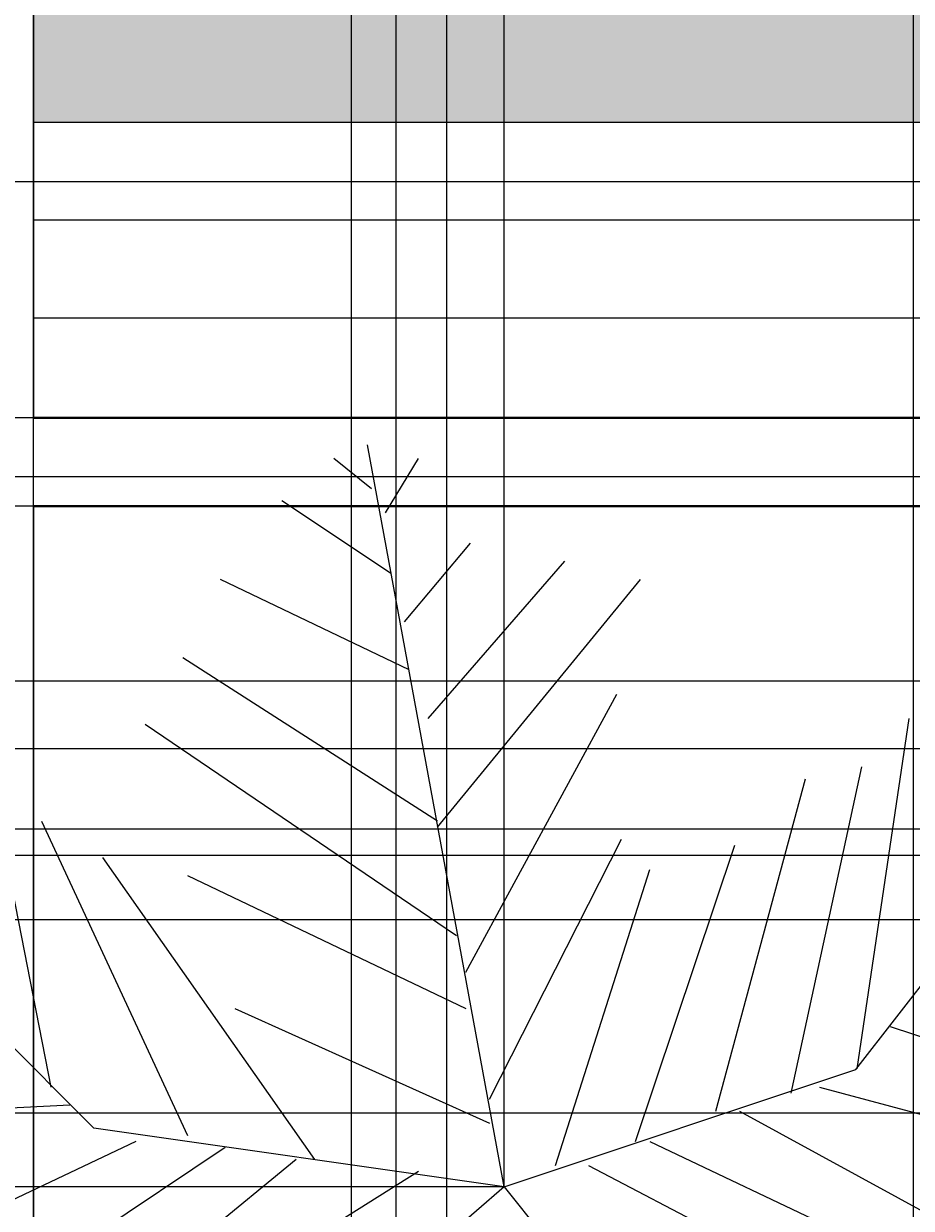
# Model space of a CAD drawing. Units: inches. Extents: x 818 to 1898, y 976 to 2364.
# Tile 64 of 96: x 1083 to 1173, y 1972 to 2093. Entities that reach past the tile are written whole.
import ezdxf

# ---------------------------------------------------------------- set-up
doc = ezdxf.new("R2010")
doc.units = ezdxf.units.IN
doc.header["$LTSCALE"] = 5
doc.header["$MEASUREMENT"] = 0
for name, color, linetype, lineweight in [('A-ANNO-DIMS', 2, 'Continuous', 18), ('A-FLOR-STRS', 7, 'Continuous', 25), ('A-WALL', 7, 'Continuous', 40), ('L-PLNT-BEDS', 94, 'Continuous', 18)]:
    doc.layers.add(name, color=color, linetype=linetype, lineweight=lineweight)
doc.layers.add('L-PLNT', color=116, linetype='Continuous', lineweight=13, true_color=0x136734)
doc.layers.add('L-PLNT-PATT', color=114, linetype='Continuous', lineweight=9, true_color=0x139b48)
doc.styles.get("Standard").update_dxf_attribs({"font": 'arial.ttf'})
doc.dimstyles.get("Standard").update_dxf_attribs({"dimtxt": 0.18, "dimasz": 0.18, "dimexe": 0.18, "dimexo": 0.0625, "dimgap": 0.09, "dimtad": 0, "dimtih": 1, "dimtoh": 1, "dimdec": 4, "dimzin": 0, "dimdsep": 46, "dimtxsty": 'Standard', "dimcen": 0.09, "dimadec": 0, "dimazin": 0, "dimtfac": 1, "dimtdec": 4, "dimtofl": 0, "dimtmove": 0, "dimatfit": 3, "dimfxl": 1, "dimtolj": 1, "dimtzin": 0, "dimarcsym": 0})

# ---------------------------------------------------------------- blocks, each defined once
blk = doc.blocks.new('PALM-DECK')
for p, q in [((74.19, 69.77), (60.24, 145.52)), ((60.66, 141.05), (56.81, 144.14)), ((62.1, 138.58), (65.47, 144.14)), ((62.58, 132.41), (51.51, 139.82)), ((64.03, 127.47), (70.77, 135.5)), ((66.43, 117.6), (80.4, 133.65)), ((64.51, 122.54), (45.25, 131.79)), ((67.4, 106.49), (88.1, 131.79)), ((67.4, 107.11), (41.4, 123.77)), ((70.29, 91.68), (85.69, 120.07)), ((110.08, 81.73), (137.98, 117.61)), ((110.24, 81.8), (115.54, 117.6)), ((69.32, 95.38), (37.55, 116.98)), ((103.5, 79.33), (110.72, 112.66)), ((95.8, 77.48), (104.95, 111.43)), ((26.96, 107.11), (41.88, 75.01)), ((72.69, 78.72), (86.17, 105.26)), ((23.11, 104.64), (27.92, 79.95)), ((87.62, 74.4), (97.73, 104.64)), ((32.33, 75.75), (4.43, 103.66)), ((54.88, 72.55), (33.22, 103.4)), ((79.43, 71.93), (89.06, 102.17)), ((41.88, 101.55), (70.29, 87.97)), ((46.7, 87.97), (72.69, 76.25)), ((113.61, 86.12), (138.16, 78.1)), ((74.19, 69.77), (110.08, 81.73)), ((106.39, 79.95), (136.24, 71.93)), ((29.85, 78.1), (4.81, 76.87)), ((98.21, 77.48), (120.83, 65.14)), ((74.19, 69.77), (32.33, 75.75)), ((36.59, 74.4), (10.59, 62.05)), ((89.06, 74.4), (115.06, 62.05)), ((45.73, 73.78), (23.59, 58.97)), ((52.96, 72.55), (34.18, 57.12)), ((82.8, 71.93), (108.8, 58.35)), ((65.47, 71.31), (45.73, 58.97)), ((74.19, 69.77), (44.29, 43.85)), ((74.19, 69.77), (98.11, 39.87))]:
    blk.add_line(p, q)
blk = doc.blocks.new('*D59')
at = {"layer": 'A-ANNO-DIMS', "color": 0, "lineweight": -2, "ltscale": 5, "transparency": 16777216}
for p, q in [((1251.64, 2300.39), (818.03, 2300.39)), ((818.21, 2300.21), (818.21, 1669.95)), ((818.21, 1039.32), (818.21, 1669.59)), ((896.05, 1039.14), (818.03, 1039.14))]:
    blk.add_line(p, q, dxfattribs=at)
at = {"layer": 'A-ANNO-DIMS', "color": 0, "ltscale": 5, "transparency": 16777216}
for points in [[(818.18, 2300.21), (818.24, 2300.21), (818.21, 2300.39)], [(818.18, 1039.32), (818.24, 1039.32), (818.21, 1039.14)]]:
    blk.add_solid(points, dxfattribs=at)
at = {"layer": 'Defpoints', "color": 0, "ltscale": 5, "transparency": 16777216}
for p in [(818.21, 2300.39), (1251.71, 2300.39), (896.11, 1039.14)]:
    blk.add_point(p, dxfattribs=at)
at = {"layer": 'A-ANNO-DIMS', "color": 0, "ltscale": 5, "transparency": 16777216, "insert": (818.21, 1669.77), "char_height": 0.18, "attachment_point": 5}
blk.add_mtext('\\A1;1261.2', dxfattribs=at)
blk = doc.blocks.new('*D61')
at = {"layer": 'A-ANNO-DIMS', "color": 0, "lineweight": -2, "ltscale": 5, "transparency": 16777216}
for p, q in [((1071.73, 1203.03), (1071.73, 2363.87)), ((1430.73, 1203.03), (1430.73, 2363.87)), ((1071.91, 2363.69), (1250.94, 2363.69)), ((1430.55, 2363.69), (1251.51, 2363.69))]:
    blk.add_line(p, q, dxfattribs=at)
at = {"layer": 'A-ANNO-DIMS', "color": 0, "ltscale": 5, "transparency": 16777216}
for points in [[(1071.91, 2363.72), (1071.91, 2363.66), (1071.73, 2363.69)], [(1430.55, 2363.72), (1430.55, 2363.66), (1430.73, 2363.69)]]:
    blk.add_solid(points, dxfattribs=at)
at = {"layer": 'Defpoints', "color": 0, "ltscale": 5, "transparency": 16777216}
for p in [(1430.73, 2363.69), (1071.73, 1202.96), (1430.73, 1202.96)]:
    blk.add_point(p, dxfattribs=at)
at = {"layer": 'A-ANNO-DIMS', "color": 0, "ltscale": 5, "transparency": 16777216, "insert": (1251.23, 2363.69), "char_height": 0.18, "attachment_point": 5}
blk.add_mtext('\\A1;359', dxfattribs=at)
blk = doc.blocks.new('*D67')
at = {"layer": 'A-ANNO-DIMS', "color": 0, "lineweight": -2, "ltscale": 5, "transparency": 16777216}
for p, q in [((1083.66, 2205.97), (818.03, 2205.97)), ((818.21, 2205.79), (818.21, 2129.71)), ((818.21, 2053.26), (818.21, 2129.34)), ((1083.66, 2053.08), (818.03, 2053.08))]:
    blk.add_line(p, q, dxfattribs=at)
at = {"layer": 'A-ANNO-DIMS', "color": 0, "ltscale": 5, "transparency": 16777216}
for points in [[(818.18, 2205.79), (818.24, 2205.79), (818.21, 2205.97)], [(818.18, 2053.26), (818.24, 2053.26), (818.21, 2053.08)]]:
    blk.add_solid(points, dxfattribs=at)
at = {"layer": 'Defpoints', "color": 0, "ltscale": 5, "transparency": 16777216}
for p in [(818.21, 2205.97), (1083.73, 2205.97), (1083.73, 2053.08)]:
    blk.add_point(p, dxfattribs=at)
at = {"layer": 'A-ANNO-DIMS', "color": 0, "ltscale": 5, "transparency": 16777216, "insert": (818.21, 2129.52), "char_height": 0.18, "attachment_point": 5}
blk.add_mtext('\\A1;152.9', dxfattribs=at)
blk = doc.blocks.new('*D73')
at = {"layer": 'A-ANNO-DIMS', "color": 0, "lineweight": -2, "ltscale": 5, "transparency": 16777216}
for p, q in [((1590.66, 2011.08), (818.03, 2011.08)), ((818.21, 2010.9), (818.21, 1996.76)), ((818.21, 1982.26), (818.21, 1996.4)), ((1590.66, 1982.08), (818.03, 1982.08))]:
    blk.add_line(p, q, dxfattribs=at)
at = {"layer": 'A-ANNO-DIMS', "color": 0, "ltscale": 5, "transparency": 16777216}
for points in [[(818.18, 2010.9), (818.24, 2010.9), (818.21, 2011.08)], [(818.18, 1982.26), (818.24, 1982.26), (818.21, 1982.08)]]:
    blk.add_solid(points, dxfattribs=at)
at = {"layer": 'Defpoints', "color": 0, "ltscale": 5, "transparency": 16777216}
for p in [(818.21, 2011.08), (1590.73, 2011.08), (1590.73, 1982.08)]:
    blk.add_point(p, dxfattribs=at)
at = {"layer": 'A-ANNO-DIMS', "color": 0, "ltscale": 5, "transparency": 16777216, "insert": (818.21, 1996.58), "char_height": 0.18, "attachment_point": 5}
blk.add_mtext('\\A1;29', dxfattribs=at)
blk = doc.blocks.new('*D82')
at = {"layer": 'A-ANNO-DIMS', "color": 0, "lineweight": -2, "ltscale": 5, "transparency": 16777216}
for p, q in [((1083.73, 1501.14), (1083.73, 2363.87)), ((1197.73, 1501.14), (1197.73, 2363.87)), ((1083.91, 2363.69), (1140.45, 2363.69)), ((1197.55, 2363.69), (1141.01, 2363.69))]:
    blk.add_line(p, q, dxfattribs=at)
at = {"layer": 'A-ANNO-DIMS', "color": 0, "ltscale": 5, "transparency": 16777216}
for points in [[(1083.91, 2363.72), (1083.91, 2363.66), (1083.73, 2363.69)], [(1197.55, 2363.72), (1197.55, 2363.66), (1197.73, 2363.69)]]:
    blk.add_solid(points, dxfattribs=at)
at = {"layer": 'Defpoints', "color": 0, "ltscale": 5, "transparency": 16777216}
for p in [(1197.73, 2363.69), (1083.73, 1501.08), (1197.73, 1501.08)]:
    blk.add_point(p, dxfattribs=at)
at = {"layer": 'A-ANNO-DIMS', "color": 0, "ltscale": 5, "transparency": 16777216, "insert": (1140.73, 2363.69), "char_height": 0.18, "attachment_point": 5}
blk.add_mtext('\\A1;114', dxfattribs=at)
blk = doc.blocks.new('*D93')
at = {"layer": 'A-ANNO-DIMS', "color": 0, "lineweight": -2, "ltscale": 5, "transparency": 16777216}
for p, q in [((1068.34, 1071.12), (1068.34, 2363.87)), ((1120.76, 1071.12), (1120.76, 2363.87)), ((1068.52, 2363.69), (1094.16, 2363.69)), ((1120.58, 2363.69), (1094.94, 2363.69))]:
    blk.add_line(p, q, dxfattribs=at)
at = {"layer": 'A-ANNO-DIMS', "color": 0, "ltscale": 5, "transparency": 16777216}
for points in [[(1068.52, 2363.72), (1068.52, 2363.66), (1068.34, 2363.69)], [(1120.58, 2363.72), (1120.58, 2363.66), (1120.76, 2363.69)]]:
    blk.add_solid(points, dxfattribs=at)
at = {"layer": 'Defpoints', "color": 0, "ltscale": 5, "transparency": 16777216}
for p in [(1120.76, 2363.69), (1068.34, 1071.06), (1120.76, 1071.06)]:
    blk.add_point(p, dxfattribs=at)
at = {"layer": 'A-ANNO-DIMS', "color": 0, "ltscale": 5, "transparency": 16777216, "insert": (1094.55, 2363.69), "char_height": 0.18, "attachment_point": 5}
blk.add_mtext('\\A1;52.42', dxfattribs=at)
blk = doc.blocks.new('*D94')
at = {"layer": 'A-ANNO-DIMS', "color": 0, "lineweight": -2, "ltscale": 5, "transparency": 16777216}
for p, q in [((1120.76, 1071.12), (1120.76, 2363.87)), ((1173.54, 1071.12), (1173.54, 2363.87)), ((1120.94, 2363.69), (1146.76, 2363.69)), ((1173.36, 2363.69), (1147.55, 2363.69))]:
    blk.add_line(p, q, dxfattribs=at)
at = {"layer": 'A-ANNO-DIMS', "color": 0, "ltscale": 5, "transparency": 16777216}
for points in [[(1120.94, 2363.72), (1120.94, 2363.66), (1120.76, 2363.69)], [(1173.36, 2363.72), (1173.36, 2363.66), (1173.54, 2363.69)]]:
    blk.add_solid(points, dxfattribs=at)
at = {"layer": 'Defpoints', "color": 0, "ltscale": 5, "transparency": 16777216}
for p in [(1173.54, 2363.69), (1120.76, 1071.06), (1173.54, 1071.06)]:
    blk.add_point(p, dxfattribs=at)
at = {"layer": 'A-ANNO-DIMS', "color": 0, "ltscale": 5, "transparency": 16777216, "insert": (1147.15, 2363.69), "char_height": 0.18, "attachment_point": 5}
blk.add_mtext('\\A1;52.78', dxfattribs=at)
blk = doc.blocks.new('*D109')
at = {"layer": 'A-ANNO-DIMS', "color": 0, "lineweight": -2, "ltscale": 5, "transparency": 16777216}
for p, q in [((1125.92, 1410.12), (1125.92, 2363.87)), ((1203.33, 1409.91), (1203.33, 2363.87)), ((1126.1, 2363.69), (1164.25, 2363.69)), ((1203.15, 2363.69), (1165, 2363.69))]:
    blk.add_line(p, q, dxfattribs=at)
at = {"layer": 'A-ANNO-DIMS', "color": 0, "ltscale": 5, "transparency": 16777216}
for points in [[(1126.1, 2363.72), (1126.1, 2363.66), (1125.92, 2363.69)], [(1203.15, 2363.72), (1203.15, 2363.66), (1203.33, 2363.69)]]:
    blk.add_solid(points, dxfattribs=at)
at = {"layer": 'Defpoints', "color": 0, "ltscale": 5, "transparency": 16777216}
for p in [(1203.33, 2363.69), (1125.92, 1410.05), (1203.33, 1409.85)]:
    blk.add_point(p, dxfattribs=at)
at = {"layer": 'A-ANNO-DIMS', "color": 0, "ltscale": 5, "transparency": 16777216, "insert": (1164.62, 2363.69), "char_height": 0.18, "attachment_point": 5}
blk.add_mtext('\\A1;77.41', dxfattribs=at)
blk = doc.blocks.new('*D123')
at = {"layer": 'A-ANNO-DIMS', "color": 0, "lineweight": -2, "ltscale": 5, "transparency": 16777216}
for p, q in [((1083.73, 2044.14), (1083.73, 2363.87)), ((1131.77, 1974.64), (1131.77, 2363.87)), ((1083.91, 2363.69), (1107.35, 2363.69)), ((1131.59, 2363.69), (1108.14, 2363.69))]:
    blk.add_line(p, q, dxfattribs=at)
at = {"layer": 'A-ANNO-DIMS', "color": 0, "ltscale": 5, "transparency": 16777216}
for points in [[(1083.91, 2363.72), (1083.91, 2363.66), (1083.73, 2363.69)], [(1131.59, 2363.72), (1131.59, 2363.66), (1131.77, 2363.69)]]:
    blk.add_solid(points, dxfattribs=at)
at = {"layer": 'Defpoints', "color": 0, "ltscale": 5, "transparency": 16777216}
for p in [(1131.77, 2363.69), (1083.73, 2044.08), (1131.77, 1974.57)]:
    blk.add_point(p, dxfattribs=at)
at = {"layer": 'A-ANNO-DIMS', "color": 0, "ltscale": 5, "transparency": 16777216, "insert": (1107.75, 2363.69), "char_height": 0.18, "attachment_point": 5}
blk.add_mtext('\\A1;48.04', dxfattribs=at)
blk = doc.blocks.new('*D124')
at = {"layer": 'A-ANNO-DIMS', "color": 0, "lineweight": -2, "ltscale": 5, "transparency": 16777216}
for p, q in [((1131.7, 1974.57), (818.03, 1974.57)), ((818.21, 1974.39), (818.21, 1884.68)), ((818.21, 1794.61), (818.21, 1884.32)), ((1138.44, 1794.43), (818.03, 1794.43))]:
    blk.add_line(p, q, dxfattribs=at)
at = {"layer": 'A-ANNO-DIMS', "color": 0, "ltscale": 5, "transparency": 16777216}
for points in [[(818.18, 1974.39), (818.24, 1974.39), (818.21, 1974.57)], [(818.18, 1794.61), (818.24, 1794.61), (818.21, 1794.43)]]:
    blk.add_solid(points, dxfattribs=at)
at = {"layer": 'Defpoints', "color": 0, "ltscale": 5, "transparency": 16777216}
for p in [(818.21, 1974.57), (1131.77, 1974.57), (1138.5, 1794.43)]:
    blk.add_point(p, dxfattribs=at)
at = {"layer": 'A-ANNO-DIMS', "color": 0, "ltscale": 5, "transparency": 16777216, "insert": (818.21, 1884.5), "char_height": 0.18, "attachment_point": 5}
blk.add_mtext('\\A1;180.14', dxfattribs=at)
blk = doc.blocks.new('*D125')
at = {"layer": 'A-ANNO-DIMS', "color": 0, "lineweight": -2, "ltscale": 5, "transparency": 16777216}
for p, q in [((1083.66, 2044.08), (818.03, 2044.08)), ((818.21, 2043.9), (818.21, 2009.51)), ((818.21, 1974.75), (818.21, 2009.14)), ((1131.7, 1974.57), (818.03, 1974.57))]:
    blk.add_line(p, q, dxfattribs=at)
at = {"layer": 'A-ANNO-DIMS', "color": 0, "ltscale": 5, "transparency": 16777216}
for points in [[(818.18, 2043.9), (818.24, 2043.9), (818.21, 2044.08)], [(818.18, 1974.75), (818.24, 1974.75), (818.21, 1974.57)]]:
    blk.add_solid(points, dxfattribs=at)
at = {"layer": 'Defpoints', "color": 0, "ltscale": 5, "transparency": 16777216}
for p in [(1083.73, 2044.08), (818.21, 1974.57), (1131.77, 1974.57)]:
    blk.add_point(p, dxfattribs=at)
at = {"layer": 'A-ANNO-DIMS', "color": 0, "ltscale": 5, "transparency": 16777216, "insert": (818.21, 2009.33), "char_height": 0.18, "attachment_point": 5}
blk.add_mtext('\\A1;69.5', dxfattribs=at)
blk = doc.blocks.new('*D126')
at = {"layer": 'A-ANNO-DIMS', "color": 0, "lineweight": -2, "ltscale": 5, "transparency": 16777216}
for p, q in [((1035.38, 1252.09), (1035.38, 2363.87)), ((1116.19, 1236.03), (1116.19, 2363.87)), ((1035.56, 2363.69), (1075.41, 2363.69)), ((1116.01, 2363.69), (1076.16, 2363.69))]:
    blk.add_line(p, q, dxfattribs=at)
at = {"layer": 'A-ANNO-DIMS', "color": 0, "ltscale": 5, "transparency": 16777216}
for points in [[(1035.56, 2363.72), (1035.56, 2363.66), (1035.38, 2363.69)], [(1116.01, 2363.72), (1116.01, 2363.66), (1116.19, 2363.69)]]:
    blk.add_solid(points, dxfattribs=at)
at = {"layer": 'Defpoints', "color": 0, "ltscale": 5, "transparency": 16777216}
for p in [(1035.38, 2363.69), (1035.38, 1252.02), (1116.19, 1235.96)]:
    blk.add_point(p, dxfattribs=at)
at = {"layer": 'A-ANNO-DIMS', "color": 0, "ltscale": 5, "transparency": 16777216, "insert": (1075.78, 2363.69), "char_height": 0.18, "attachment_point": 5}
blk.add_mtext('\\A1;80.81', dxfattribs=at)
blk = doc.blocks.new('*D140')
at = {"layer": 'A-ANNO-DIMS', "color": 0, "lineweight": -2, "ltscale": 5, "transparency": 16777216}
for p, q in [((1083.73, 2053.14), (1083.73, 2363.87)), ((1218.11, 2083.32), (1218.11, 2363.87)), ((1083.91, 2363.69), (1150.46, 2363.69)), ((1217.93, 2363.69), (1151.37, 2363.69))]:
    blk.add_line(p, q, dxfattribs=at)
at = {"layer": 'A-ANNO-DIMS', "color": 0, "ltscale": 5, "transparency": 16777216}
for points in [[(1083.91, 2363.72), (1083.91, 2363.66), (1083.73, 2363.69)], [(1217.93, 2363.72), (1217.93, 2363.66), (1218.11, 2363.69)]]:
    blk.add_solid(points, dxfattribs=at)
at = {"layer": 'Defpoints', "color": 0, "ltscale": 5, "transparency": 16777216}
for p in [(1218.11, 2363.69), (1218.11, 2083.26), (1083.73, 2053.08)]:
    blk.add_point(p, dxfattribs=at)
at = {"layer": 'A-ANNO-DIMS', "color": 0, "ltscale": 5, "transparency": 16777216, "insert": (1150.92, 2363.69), "char_height": 0.18, "attachment_point": 5}
blk.add_mtext('\\A1;134.39', dxfattribs=at)
blk = doc.blocks.new('*D146')
at = {"layer": 'A-ANNO-DIMS', "color": 0, "lineweight": -2, "ltscale": 5, "transparency": 16777216}
for p, q in [((1197.33, 2122.38), (818.03, 2122.38)), ((818.21, 2122.2), (818.21, 2087.91)), ((818.21, 2053.26), (818.21, 2087.55)), ((1083.66, 2053.08), (818.03, 2053.08))]:
    blk.add_line(p, q, dxfattribs=at)
at = {"layer": 'A-ANNO-DIMS', "color": 0, "ltscale": 5, "transparency": 16777216}
for points in [[(818.18, 2122.2), (818.24, 2122.2), (818.21, 2122.38)], [(818.18, 2053.26), (818.24, 2053.26), (818.21, 2053.08)]]:
    blk.add_solid(points, dxfattribs=at)
at = {"layer": 'Defpoints', "color": 0, "ltscale": 5, "transparency": 16777216}
for p in [(1197.39, 2122.38), (818.21, 2053.08), (1083.73, 2053.08)]:
    blk.add_point(p, dxfattribs=at)
at = {"layer": 'A-ANNO-DIMS', "color": 0, "ltscale": 5, "transparency": 16777216, "insert": (818.21, 2087.73), "char_height": 0.18, "attachment_point": 5}
blk.add_mtext('\\A1;69.3', dxfattribs=at)
blk = doc.blocks.new('*D207')
at = {"layer": 'A-ANNO-DIMS', "color": 0, "lineweight": -2, "ltscale": 5, "transparency": 16777216}
for p, q in [((1590.66, 2044.08), (818.03, 2044.08)), ((818.21, 2043.9), (818.21, 2027.76)), ((818.21, 2011.26), (818.21, 2027.4)), ((1590.66, 2011.08), (818.03, 2011.08))]:
    blk.add_line(p, q, dxfattribs=at)
at = {"layer": 'A-ANNO-DIMS', "color": 0, "ltscale": 5, "transparency": 16777216}
for points in [[(818.18, 2043.9), (818.24, 2043.9), (818.21, 2044.08)], [(818.18, 2011.26), (818.24, 2011.26), (818.21, 2011.08)]]:
    blk.add_solid(points, dxfattribs=at)
at = {"layer": 'Defpoints', "color": 0, "ltscale": 5, "transparency": 16777216}
for p in [(818.21, 2044.08), (1590.73, 2044.08), (1590.73, 2011.08)]:
    blk.add_point(p, dxfattribs=at)
at = {"layer": 'A-ANNO-DIMS', "color": 0, "ltscale": 5, "transparency": 16777216, "insert": (818.21, 2027.58), "char_height": 0.18, "attachment_point": 5}
blk.add_mtext('\\A1;33', dxfattribs=at)
blk = doc.blocks.new('*D232')
at = {"layer": 'A-ANNO-DIMS', "color": 0, "lineweight": -2, "ltscale": 5, "transparency": 16777216}
for p, q in [((1303.87, 2008.39), (818.03, 2008.39)), ((818.21, 2008.21), (818.21, 1980.9)), ((818.21, 1953.22), (818.21, 1980.53)), ((1303.87, 1953.04), (818.03, 1953.04))]:
    blk.add_line(p, q, dxfattribs=at)
at = {"layer": 'A-ANNO-DIMS', "color": 0, "ltscale": 5, "transparency": 16777216}
for points in [[(818.18, 2008.21), (818.24, 2008.21), (818.21, 2008.39)], [(818.18, 1953.22), (818.24, 1953.22), (818.21, 1953.04)]]:
    blk.add_solid(points, dxfattribs=at)
at = {"layer": 'Defpoints', "color": 0, "ltscale": 5, "transparency": 16777216}
for p in [(818.21, 2008.39), (1303.93, 2008.39), (1303.93, 1953.04)]:
    blk.add_point(p, dxfattribs=at)
at = {"layer": 'A-ANNO-DIMS', "color": 0, "ltscale": 5, "transparency": 16777216, "insert": (818.21, 1980.72), "char_height": 0.18, "attachment_point": 5}
blk.add_mtext('\\A1;55.35', dxfattribs=at)
blk = doc.blocks.new('*D234')
at = {"layer": 'A-ANNO-DIMS', "color": 0, "lineweight": -2, "ltscale": 5, "transparency": 16777216}
for p, q in [((1267.66, 2044.08), (818.03, 2044.08)), ((818.21, 2043.9), (818.21, 2026.42)), ((818.21, 2008.57), (818.21, 2026.05)), ((1303.87, 2008.39), (818.03, 2008.39))]:
    blk.add_line(p, q, dxfattribs=at)
at = {"layer": 'A-ANNO-DIMS', "color": 0, "ltscale": 5, "transparency": 16777216}
for points in [[(818.18, 2043.9), (818.24, 2043.9), (818.21, 2044.08)], [(818.18, 2008.57), (818.24, 2008.57), (818.21, 2008.39)]]:
    blk.add_solid(points, dxfattribs=at)
at = {"layer": 'Defpoints', "color": 0, "ltscale": 5, "transparency": 16777216}
for p in [(818.21, 2044.08), (1267.73, 2044.08), (1303.93, 2008.39)]:
    blk.add_point(p, dxfattribs=at)
at = {"layer": 'A-ANNO-DIMS', "color": 0, "ltscale": 5, "transparency": 16777216, "insert": (818.21, 2026.23), "char_height": 0.18, "attachment_point": 5}
blk.add_mtext('\\A1;35.69', dxfattribs=at)
blk = doc.blocks.new('*D237')
at = {"layer": 'A-ANNO-DIMS', "color": 0, "lineweight": -2, "ltscale": 5, "transparency": 16777216}
for p, q in [((1310.85, 2026.21), (818.03, 2026.21)), ((818.21, 2026.03), (818.21, 2014.2)), ((818.21, 2002), (818.21, 2013.83)), ((1314.2, 2001.82), (818.03, 2001.82))]:
    blk.add_line(p, q, dxfattribs=at)
at = {"layer": 'A-ANNO-DIMS', "color": 0, "ltscale": 5, "transparency": 16777216}
for points in [[(818.18, 2026.03), (818.24, 2026.03), (818.21, 2026.21)], [(818.18, 2002), (818.24, 2002), (818.21, 2001.82)]]:
    blk.add_solid(points, dxfattribs=at)
at = {"layer": 'Defpoints', "color": 0, "ltscale": 5, "transparency": 16777216}
for p in [(1310.91, 2026.21), (818.21, 2001.82), (1314.26, 2001.82)]:
    blk.add_point(p, dxfattribs=at)
at = {"layer": 'A-ANNO-DIMS', "color": 0, "ltscale": 5, "transparency": 16777216, "insert": (818.21, 2014.02), "char_height": 0.18, "attachment_point": 5}
blk.add_mtext('\\A1;24.383', dxfattribs=at)
blk = doc.blocks.new('*D248')
at = {"layer": 'A-ANNO-DIMS', "color": 0, "lineweight": -2, "ltscale": 5, "transparency": 16777216}
for p, q in [((1258.66, 2019.29), (818.03, 2019.29)), ((818.21, 2019.11), (818.21, 1974.29)), ((818.21, 1929.1), (818.21, 1973.92)), ((1258.66, 1928.92), (818.03, 1928.92))]:
    blk.add_line(p, q, dxfattribs=at)
at = {"layer": 'A-ANNO-DIMS', "color": 0, "ltscale": 5, "transparency": 16777216}
for points in [[(818.18, 2019.11), (818.24, 2019.11), (818.21, 2019.29)], [(818.18, 1929.1), (818.24, 1929.1), (818.21, 1928.92)]]:
    blk.add_solid(points, dxfattribs=at)
at = {"layer": 'Defpoints', "color": 0, "ltscale": 5, "transparency": 16777216}
for p in [(818.21, 2019.29), (1258.73, 2019.29), (1258.73, 1928.92)]:
    blk.add_point(p, dxfattribs=at)
at = {"layer": 'A-ANNO-DIMS', "color": 0, "ltscale": 5, "transparency": 16777216, "insert": (818.21, 1974.1), "char_height": 0.18, "attachment_point": 5}
blk.add_mtext('\\A1;90.37', dxfattribs=at)
blk = doc.blocks.new('*D257')
at = {"layer": 'A-ANNO-DIMS', "color": 0, "lineweight": -2, "ltscale": 5, "transparency": 16777216}
for p, q in [((1399.57, 2077.19), (818.03, 2077.19)), ((818.21, 2077.01), (818.21, 2065.31)), ((818.21, 2053.26), (818.21, 2064.95)), ((1399.57, 2053.08), (818.03, 2053.08))]:
    blk.add_line(p, q, dxfattribs=at)
at = {"layer": 'A-ANNO-DIMS', "color": 0, "ltscale": 5, "transparency": 16777216}
for points in [[(818.18, 2077.01), (818.24, 2077.01), (818.21, 2077.19)], [(818.18, 2053.26), (818.24, 2053.26), (818.21, 2053.08)]]:
    blk.add_solid(points, dxfattribs=at)
at = {"layer": 'Defpoints', "color": 0, "ltscale": 5, "transparency": 16777216}
for p in [(818.21, 2077.19), (1399.64, 2077.19), (1399.64, 2053.08)]:
    blk.add_point(p, dxfattribs=at)
at = {"layer": 'A-ANNO-DIMS', "color": 0, "ltscale": 5, "transparency": 16777216, "insert": (818.21, 2065.13), "char_height": 0.18, "attachment_point": 5}
blk.add_mtext('\\A1;24.11', dxfattribs=at)
blk = doc.blocks.new('*D266')
at = {"layer": 'A-ANNO-DIMS', "color": 0, "lineweight": -2, "ltscale": 5, "transparency": 16777216}
for p, q in [((1780.44, 2053.08), (818.03, 2053.08)), ((818.21, 2052.9), (818.21, 2050.26)), ((818.21, 2047.26), (818.21, 2049.9)), ((1780.44, 2047.08), (818.03, 2047.08))]:
    blk.add_line(p, q, dxfattribs=at)
at = {"layer": 'A-ANNO-DIMS', "color": 0, "ltscale": 5, "transparency": 16777216}
for points in [[(818.18, 2052.9), (818.24, 2052.9), (818.21, 2053.08)], [(818.18, 2047.26), (818.24, 2047.26), (818.21, 2047.08)]]:
    blk.add_solid(points, dxfattribs=at)
at = {"layer": 'Defpoints', "color": 0, "ltscale": 5, "transparency": 16777216}
for p in [(1780.5, 2053.08), (818.21, 2047.08), (1780.5, 2047.08)]:
    blk.add_point(p, dxfattribs=at)
at = {"layer": 'A-ANNO-DIMS', "color": 0, "ltscale": 5, "transparency": 16777216, "insert": (818.21, 2050.08), "char_height": 0.18, "attachment_point": 5}
blk.add_mtext('\\A1;6', dxfattribs=at)

msp = doc.modelspace()

# ---------------------------------------------------------------- hatches: boundary and pattern name
at = {"layer": 'L-PLNT-PATT', "ltscale": 5}
h = msp.add_hatch(color=256, dxfattribs=at)
h.dxf.hatch_style = 1
h.paths.add_polyline_path([(1789.7173, 2205.9709), (1083.7251, 2205.9709), (1083.7251, 2083.2623), (1218.1114, 2083.2623), (1218.1114, 2053.0782), (1390.6356, 2053.0782), (1390.6356, 2081.1881), (1399.6356, 2081.1881), (1413.02, 2081.1881), (1422.02, 2081.1881), (1422.02, 2053.0782), (1676.6446, 2053.0782), (1676.6446, 2081.1881), (1714.7252, 2081.1881), (1714.7252, 2081.6235), (1789.7173, 2081.6235)])
h.paths.add_polyline_path([(1388.6037, 2145.2461), (1388.6037, 2122.3767), (1373.4756, 2122.3767), (1373.4756, 2145.2461)], flags=16)
h.paths.add_polyline_path([(1408.6922, 2145.2461), (1423.8203, 2145.2461), (1423.8203, 2122.3767), (1408.6922, 2122.3767)], flags=16)
h.paths.add_polyline_path([(1353.3871, 2155.7839), (1353.3871, 2122.3767), (1338.259, 2122.3767), (1338.259, 2155.7839)], flags=16)
h.paths.add_polyline_path([(1443.9089, 2158.4222), (1459.037, 2158.4222), (1459.037, 2122.3767), (1443.9089, 2122.3767)], flags=16)
h.paths.add_polyline_path([(1318.1705, 2145.2461), (1318.1705, 2122.3767), (1303.0424, 2122.3767), (1303.0424, 2145.2461)], flags=16)
h.paths.add_polyline_path([(1479.1255, 2145.2461), (1494.2536, 2145.2461), (1494.2536, 2122.3767), (1479.1255, 2122.3767)], flags=16)
h.paths.add_polyline_path([(1282.9539, 2145.2461), (1282.9539, 2122.3767), (1267.8258, 2122.3767), (1267.8258, 2145.2461)], flags=16)
h.paths.add_polyline_path([(1514.3421, 2145.2461), (1529.4702, 2145.2461), (1529.4702, 2122.3767), (1514.3421, 2122.3767)], flags=16)
h.paths.add_polyline_path([(1247.7373, 2159.4296), (1247.7373, 2122.3767), (1232.6091, 2122.3767), (1232.6091, 2159.4296)], flags=16)
h.paths.add_polyline_path([(1549.5587, 2156.9246), (1564.6868, 2156.9246), (1564.6868, 2122.3767), (1549.5587, 2122.3767)], flags=16)
h.paths.add_polyline_path([(1212.5206, 2145.2461), (1212.5206, 2122.3767), (1197.3925, 2122.3767), (1197.3925, 2145.2461)], flags=16)
h.paths.add_polyline_path([(1584.7753, 2145.2461), (1599.9034, 2145.2461), (1599.9034, 2122.3767), (1584.7753, 2122.3767)], flags=16)
h.paths.add_polyline_path([(1185.1073, 2104.7786), (1190.6407, 2104.7786), (1185.1073, 2098.2505), (1179.5738, 2104.7786)], flags=16)
h.paths.add_polyline_path([(1619.9919, 2145.2461), (1635.1201, 2145.2461), (1635.1201, 2122.3767), (1619.9919, 2122.3767)], flags=16)
h.paths.add_polyline_path([(1655.2086, 2156.1761), (1670.3367, 2156.1761), (1670.3367, 2122.3767), (1655.2086, 2122.3767)], flags=16)
h.paths.add_polyline_path([(1686.5992, 2145.2461), (1701.7273, 2145.2461), (1701.7273, 2122.3767), (1686.5992, 2122.3767)], flags=16)
h.paths.add_polyline_path([(1715.7616, 2145.2461), (1730.8897, 2145.2461), (1730.8897, 2122.3767), (1715.7616, 2122.3767)], flags=16)
h.paths.add_polyline_path([(1753.1652, 2145.2461), (1776.3312, 2145.2461), (1776.3312, 2115.6891), (1753.1652, 2115.6891)], flags=16)
h.paths.add_polyline_path([(1191.4331, 2146.5159), (1176.7891, 2146.5159), (1176.7891, 2134.1516), (1191.4331, 2134.1516)], flags=24)

# ---------------------------------------------------------------- linework, layer by layer
at = {"layer": 'A-FLOR-STRS', "ltscale": 5}
for p, q in [((1218.1114, 2083.2623), (1083.7251, 2083.2623)), ((1208.1114, 2073.2623), (1083.7251, 2073.2623)), ((1198.1114, 2063.2623), (1083.7251, 2063.2623)), ((1083.7251, 2063.2623), (1083.7251, 2053.0782)), ((1083.7251, 2053.0782), (1198.1114, 2053.0782))]:
    msp.add_line(p, q, dxfattribs=at)
at = {"layer": 'A-WALL'}
for p, q in [((1083.7251, 2053.0782), (1390.6356, 2053.0782)), ((1083.7251, 2044.0782), (1214.6577, 2044.0782))]:
    msp.add_line(p, q, dxfattribs=at)
at = {"layer": 'L-PLNT-BEDS'}
for p, q in [((1083.7251, 2205.9709), (1083.7251, 2053.0782)), ((1083.7251, 2044.0782), (1083.7251, 1211.9642))]:
    msp.add_line(p, q, dxfattribs=at)

# ---------------------------------------------------------------- block references
at = {"layer": 'L-PLNT'}
msp.add_blockref('PALM-DECK', (1057.571, 1904.8049), dxfattribs=at)

# ---------------------------------------------------------------- dimensions: what is measured, and where the dimension line sits
at = {"layer": 'A-ANNO-DIMS', "ltscale": 5}
for base, p1, p2, override, picture, middle in [((1035.3768, 2363.6929), (1116.1882, 1235.9642), (1035.3768, 1252.0242), {"dimdec": 2, "dimlfac": 1, "dimrnd": 0, "dimzin": 0, "dimdsep": 46, "dimlunit": 2}, '*D126', (1075.7825, 2363.6929)), ((1120.7618, 2363.6929), (1068.3377, 1071.0552), (1120.7618, 1071.0552), {"dimdec": 2, "dimlfac": 1, "dimrnd": 0, "dimzin": 0, "dimdsep": 46, "dimlunit": 2}, '*D93', (1094.5497, 2363.6929)), ((1430.7251, 2363.6929), (1071.7251, 1202.9642), (1430.7251, 1202.9642), {"dimdec": 0, "dimlfac": 1, "dimrnd": 0, "dimzin": 0, "dimdsep": 46, "dimlunit": 2}, '*D61', (1251.2251, 2363.6929)), ((1197.7251, 2363.6929), (1083.7251, 1501.0782), (1197.7251, 1501.0782), {"dimdec": 0, "dimlfac": 1, "dimrnd": 0, "dimzin": 0, "dimdsep": 46, "dimlunit": 2}, '*D82', (1140.7251, 2363.6929)), ((1131.7651, 2363.6929), (1083.7251, 2044.0782), (1131.7651, 1974.5735), {"dimdec": 2, "dimlfac": 1, "dimrnd": 0, "dimzin": 0, "dimdsep": 46, "dimlunit": 2}, '*D123', (1107.7451, 2363.6929)), ((1218.1114, 2363.6929), (1083.7251, 2053.0782), (1218.1114, 2083.2623), {"dimdec": 2, "dimlfac": 1, "dimrnd": 0, "dimzin": 0, "dimdsep": 46, "dimlunit": 2}, '*D140', (1150.9183, 2363.6929)), ((1173.5418, 2363.6929), (1120.7618, 1071.0552), (1173.5418, 1071.0552), {"dimdec": 2, "dimlfac": 1, "dimrnd": 0, "dimzin": 0, "dimdsep": 46, "dimlunit": 2}, '*D94', (1147.1518, 2363.6929)), ((1203.3292, 2363.6929), (1125.9172, 1410.0547), (1203.3292, 1409.8484), {"dimdec": 2, "dimlfac": 1, "dimrnd": 0, "dimzin": 0, "dimdsep": 46, "dimlunit": 2}, '*D109', (1164.6232, 2363.6929))]:
    dim = msp.add_linear_dim(base=base, p1=p1, p2=p2, dimstyle='Standard', override=override, dxfattribs=at)
    dim.commit()
    dim.dimension.update_dxf_attribs({"geometry": picture, "text_midpoint": middle})
for base, p1, p2, override, picture, middle in [((818.2059, 2300.3929), (896.1138, 1039.1433), (1251.7057, 2300.3929), {"dimdec": 1, "dimlfac": 1, "dimrnd": 0, "dimzin": 0, "dimdsep": 46, "dimlunit": 2}, '*D59', (818.2059, 1669.7681)), ((818.2059, 2205.9709), (1083.7251, 2053.0782), (1083.7251, 2205.9709), {"dimdec": 1, "dimlfac": 1, "dimrnd": 0, "dimzin": 0, "dimdsep": 46, "dimlunit": 2}, '*D67', (818.2059, 2129.5246)), ((818.2059, 2053.0782), (1197.3925, 2122.3767), (1083.7251, 2053.0782), {"dimdec": 1, "dimlfac": 1, "dimrnd": 0, "dimzin": 0, "dimdsep": 46, "dimlunit": 2}, '*D146', (818.2059, 2087.7275)), ((818.2059, 2077.1881), (1399.6356, 2053.0782), (1399.6356, 2077.1881), {"dimdec": 2, "dimlfac": 1, "dimrnd": 0, "dimzin": 0, "dimdsep": 46, "dimlunit": 2}, '*D257', (818.2059, 2065.1332)), ((818.2059, 2047.0782), (1780.5019, 2053.0782), (1780.5019, 2047.0782), {"dimdec": 0, "dimlfac": 1, "dimrnd": 0, "dimzin": 0, "dimdsep": 46, "dimlunit": 2}, '*D266', (818.2059, 2050.0782)), ((818.2059, 2044.0782), (1303.9314, 2008.3917), (1267.7251, 2044.0782), {"dimdec": 2, "dimlfac": 1, "dimrnd": 0, "dimzin": 0, "dimdsep": 46, "dimlunit": 2}, '*D234', (818.2059, 2026.235)), ((818.2059, 1974.5735), (1083.7251, 2044.0782), (1131.7651, 1974.5735), {"dimdec": 1, "dimlfac": 1, "dimrnd": 0, "dimzin": 0, "dimdsep": 46, "dimlunit": 2}, '*D125', (818.2059, 2009.3258)), ((818.2059, 2044.0782), (1590.7251, 2011.0782), (1590.7251, 2044.0782), {"dimdec": 0, "dimlfac": 1, "dimrnd": 0, "dimzin": 0, "dimdsep": 46, "dimlunit": 2}, '*D207', (818.2059, 2027.5782)), ((818.2059, 2001.8247), (1310.9077, 2026.2074), (1314.2595, 2001.8247), {"dimdec": 3, "dimlfac": 1, "dimrnd": 0, "dimzin": 0, "dimdsep": 46, "dimlunit": 2}, '*D237', (818.2059, 2014.016)), ((818.2059, 2019.2871), (1258.7251, 1928.9218), (1258.7251, 2019.2871), {"dimdec": 2, "dimlfac": 1, "dimrnd": 0, "dimzin": 0, "dimdsep": 46, "dimlunit": 2}, '*D248', (818.2059, 1974.1044)), ((818.2059, 2011.0782), (1590.7251, 1982.0782), (1590.7251, 2011.0782), {"dimdec": 0, "dimlfac": 1, "dimrnd": 0, "dimzin": 0, "dimdsep": 46, "dimlunit": 2}, '*D73', (818.2059, 1996.5782)), ((818.2059, 2008.3917), (1303.9314, 1953.0408), (1303.9314, 2008.3917), {"dimdec": 2, "dimlfac": 1, "dimrnd": 0, "dimzin": 0, "dimdsep": 46, "dimlunit": 2}, '*D232', (818.2059, 1980.7163)), ((818.2059, 1974.5735), (1138.5041, 1794.4325), (1131.7651, 1974.5735), {"dimdec": 2, "dimlfac": 1, "dimrnd": 0, "dimzin": 0, "dimdsep": 46, "dimlunit": 2}, '*D124', (818.2059, 1884.503))]:
    dim = msp.add_linear_dim(base=base, p1=p1, p2=p2, angle=90, dimstyle='Standard', override=override, dxfattribs=at)
    dim.commit()
    dim.dimension.update_dxf_attribs({"geometry": picture, "text_midpoint": middle})

doc.saveas('drawing.dxf')
